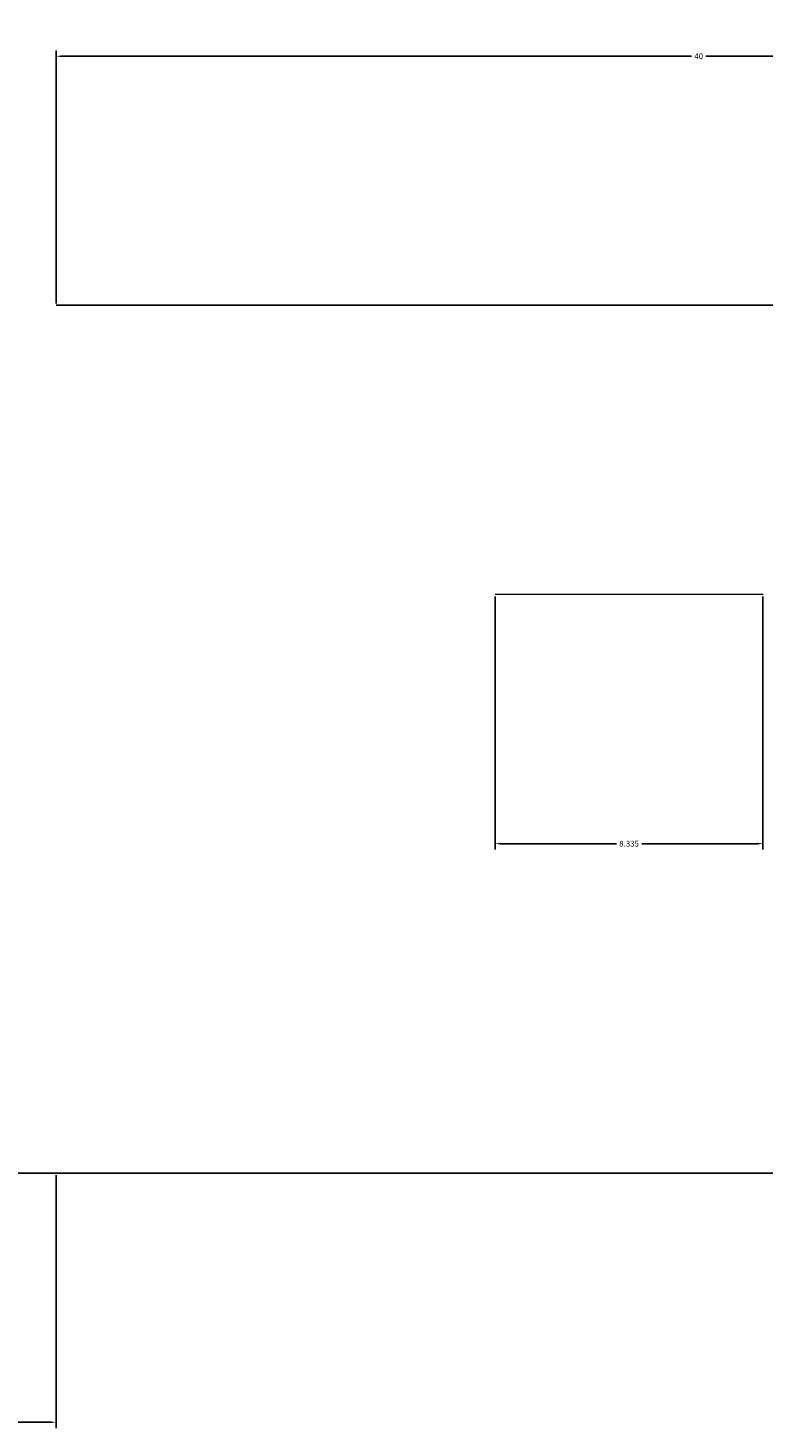
# Model space of a CAD drawing. Units: millimetres. Extents: x 223 to 381, y -8 to 62.
# Tile 3 of 5: x 332 to 355, y -8 to 36. Entities that reach past the tile are written whole.
import ezdxf

# ---------------------------------------------------------------- set-up
doc = ezdxf.new("R2010")
doc.units = ezdxf.units.MM
doc.layers.add('M-CONS', color=8, linetype='Continuous', lineweight=13)
doc.layers.add('M-DIMS', color=2, linetype='Continuous', lineweight=18)
doc.styles.get("Standard").update_dxf_attribs({"font": 'arial.ttf'})
doc.dimstyles.get("Standard").update_dxf_attribs({"dimtxt": 0.18, "dimasz": 0.18, "dimexe": 0.18, "dimexo": 0.0625, "dimgap": 0.09, "dimtad": 0, "dimtih": 1, "dimtoh": 1, "dimdec": 4, "dimzin": 0, "dimdsep": 46, "dimtxsty": 'Standard', "dimcen": 0.09, "dimadec": 0, "dimazin": 0, "dimtfac": 1, "dimtdec": 4, "dimtofl": 0, "dimtmove": 0, "dimatfit": 3, "dimfxl": 1, "dimtolj": 1, "dimtzin": 0, "dimarcsym": 0})

# ---------------------------------------------------------------- blocks, each defined once
blk = doc.blocks.new('*D1')
at = {"layer": 'Defpoints', "color": 0, "transparency": 16777216}
for p in [(372.659, 61.75), (372.659, 27), (230.659, 0)]:
    blk.add_point(p, dxfattribs=at)
at = {"layer": 'M-DIMS', "color": 0, "lineweight": -2, "transparency": 16777216}
for p, q in [((230.659, 0.062), (230.659, 61.93)), ((372.659, 27.062), (372.659, 61.93)), ((230.839, 61.75), (301.38, 61.75)), ((372.479, 61.75), (301.939, 61.75))]:
    blk.add_line(p, q, dxfattribs=at)
at = {"layer": 'M-DIMS', "color": 0, "transparency": 16777216}
for points in [[(230.839, 61.78), (230.839, 61.72), (230.659, 61.75)], [(372.479, 61.78), (372.479, 61.72), (372.659, 61.75)]]:
    blk.add_solid(points, dxfattribs=at)
at = {"layer": 'M-DIMS', "color": 0, "transparency": 16777216, "insert": (301.659, 61.75), "char_height": 0.18, "attachment_point": 5}
blk.add_mtext('\\A1;142', dxfattribs=at)
blk = doc.blocks.new('*D6')
at = {"layer": 'Defpoints', "color": 0, "transparency": 16777216}
for p in [(294.659, 0), (332.659, 0), (332.659, -7.75)]:
    blk.add_point(p, dxfattribs=at)
at = {"layer": 'M-DIMS', "color": 0, "lineweight": -2, "transparency": 16777216}
for p, q in [((294.659, -0.062), (294.659, -7.93)), ((332.659, -0.062), (332.659, -7.93)), ((294.839, -7.75), (313.44, -7.75)), ((332.479, -7.75), (313.878, -7.75))]:
    blk.add_line(p, q, dxfattribs=at)
at = {"layer": 'M-DIMS', "color": 0, "transparency": 16777216}
for points in [[(294.839, -7.72), (294.839, -7.78), (294.659, -7.75)], [(332.479, -7.72), (332.479, -7.78), (332.659, -7.75)]]:
    blk.add_solid(points, dxfattribs=at)
at = {"layer": 'M-DIMS', "color": 0, "transparency": 16777216, "insert": (313.659, -7.75), "char_height": 0.18, "attachment_point": 5}
blk.add_mtext('\\A1;38', dxfattribs=at)
blk = doc.blocks.new('*D8')
at = {"layer": 'Defpoints', "color": 0, "transparency": 16777216}
for p in [(372.659, 34.75), (332.659, 27), (372.659, 27)]:
    blk.add_point(p, dxfattribs=at)
at = {"layer": 'M-DIMS', "color": 0, "lineweight": -2, "transparency": 16777216}
for p, q in [((332.659, 27.062), (332.659, 34.93)), ((372.659, 27.062), (372.659, 34.93)), ((332.839, 34.75), (352.437, 34.75)), ((372.479, 34.75), (352.881, 34.75))]:
    blk.add_line(p, q, dxfattribs=at)
at = {"layer": 'M-DIMS', "color": 0, "transparency": 16777216}
for points in [[(332.839, 34.78), (332.839, 34.72), (332.659, 34.75)], [(372.479, 34.78), (372.479, 34.72), (372.659, 34.75)]]:
    blk.add_solid(points, dxfattribs=at)
at = {"layer": 'M-DIMS', "color": 0, "transparency": 16777216, "insert": (352.659, 34.75), "char_height": 0.18, "attachment_point": 5}
blk.add_mtext('\\A1;40', dxfattribs=at)
blk = doc.blocks.new('*D9')
at = {"layer": 'Defpoints', "color": 0, "transparency": 16777216}
for p in [(346.324, 18), (354.659, 18), (346.324, 10.25)]:
    blk.add_point(p, dxfattribs=at)
at = {"layer": 'M-DIMS', "color": 0, "lineweight": -2, "transparency": 16777216}
for p, q in [((346.324, 17.938), (346.324, 10.07)), ((354.659, 17.938), (354.659, 10.07)), ((346.504, 10.25), (350.097, 10.25)), ((354.479, 10.25), (350.886, 10.25))]:
    blk.add_line(p, q, dxfattribs=at)
at = {"layer": 'M-DIMS', "color": 0, "transparency": 16777216}
for points in [[(346.504, 10.28), (346.504, 10.22), (346.324, 10.25)], [(354.479, 10.28), (354.479, 10.22), (354.659, 10.25)]]:
    blk.add_solid(points, dxfattribs=at)
at = {"layer": 'M-DIMS', "color": 0, "transparency": 16777216, "insert": (350.492, 10.25), "char_height": 0.18, "attachment_point": 5}
blk.add_mtext('\\A1;8.335', dxfattribs=at)

msp = doc.modelspace()

# ---------------------------------------------------------------- linework, layer by layer
at = {"layer": 'M-CONS', "extrusion": (0, -1, 0)}
for p, q in [((354.6592, 18, 63.6363), (346.324, 18, 63.6363)), ((260.6592, 0, 97.6363), (332.6592, 0, 97.6363)), ((354.6592, 0, 85.6363), (294.6592, 0, 85.6363)), ((332.6592, 0, 97.6363), (332.6592, 0, 103.6363)), ((332.6592, 0, 103.6363), (372.6592, 0, 103.6363)), ((372.6592, 0, 63.6363), (354.6592, 0, 63.6363)), ((354.6592, 0, 63.6363), (354.6592, 0, 85.6363))]:
    msp.add_line(p, q, dxfattribs=at)
at = {"layer": 'M-CONS'}
msp.add_polyline3d([(332.6592, 27, 103.6363), (372.6592, 27, 143.6363), (372.6592, 27, 103.6363)], close=True, dxfattribs=at)

# ---------------------------------------------------------------- dimensions: what is measured, and where the dimension line sits
at = {"layer": 'M-DIMS'}
for base, p1, p2, picture, middle in [((372.6592, 61.75), (230.6592, 0), (372.6592, 27), '*D1', (301.6592, 61.75)), ((372.6592, 34.75), (332.6592, 27), (372.6592, 27), '*D8', (352.6592, 34.75)), ((332.6592, -7.75), (294.6592, 0), (332.6592, 0), '*D6', (313.6592, -7.75))]:
    dim = msp.add_linear_dim(base=base, p1=p1, p2=p2, dimstyle='Standard', override={"dimdec": 0, "dimlfac": 1, "dimrnd": 0, "dimzin": 0, "dimdsep": 46, "dimlunit": 2}, dxfattribs=at)
    dim.commit()
    dim.dimension.update_dxf_attribs({"geometry": picture, "text_midpoint": middle})
dim = msp.add_linear_dim(base=(346.324, 10.25), p1=(354.6592, 18), p2=(346.324, 18), angle=180, dimstyle='Standard', override={"dimdec": 3, "dimlfac": 1, "dimrnd": 0, "dimzin": 0, "dimdsep": 46, "dimlunit": 2}, dxfattribs=at)
dim.commit()
dim.dimension.update_dxf_attribs({"geometry": '*D9', "text_midpoint": (350.4916, 10.25)})

doc.saveas('drawing.dxf')
